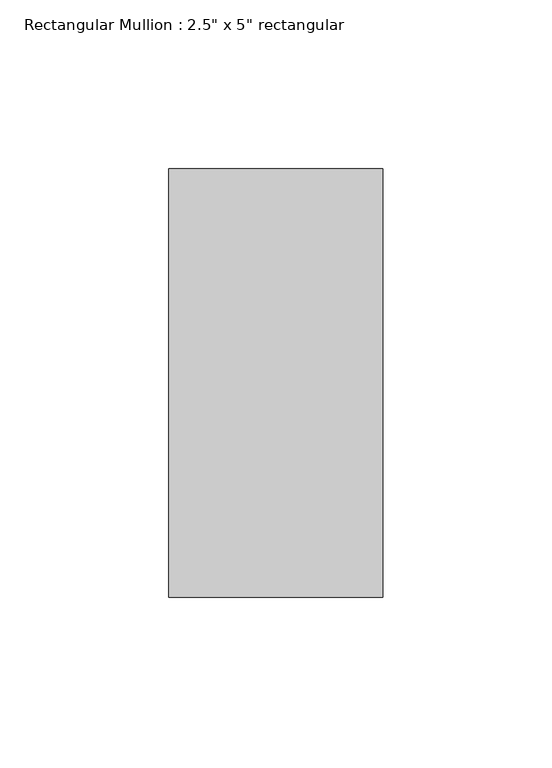
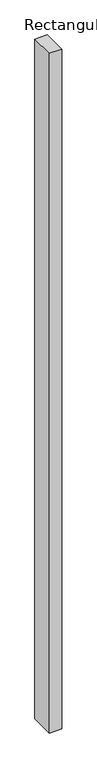
"""IFC4 building model written with IfcOpenShell, lengths in millimetres: member geometry."""

from ifc_helpers import new_model, si_unit, frame, origin, place, context, project, spatial, polyline, outline, extrude, source, transform, mapped, element, save


def member_47c71a51(model_context):
    return source(origin(), model_context, "Body", "SweptSolid", [
        extrude(outline(polyline([(0.0, 63.5), (0.0, -63.5), (-63.5, -63.5), (-63.5, 63.5), (0.0, 63.5)])), frame((0.0, 0.0, -3642.0483533), z_axis=(0.0, 0.0, 1.0), x_axis=(1.0, 0.0, 0.0)), (0.0, 0.0, 1.0), 3642.0483533),
    ])


if __name__ == "__main__":
    model = new_model("IFC4")
    model_context = context("Model", 3, world=origin())
    ifc_project = project(units=[si_unit("LENGTHUNIT", "METRE", prefix="MILLI")], contexts=[model_context])
    site = spatial("IfcSite", under=ifc_project)
    building = spatial("IfcBuilding", under=site)
    placement = place(None, origin())
    member_shape = member_47c71a51(model_context)
    element("IfcMember", 1, ObjectType="Rectangular Mullion : 2.5\" x 5\" rectangular", at=placement, inside=building, context=model_context, shape_type="MappedRepresentation", body=[
        mapped(member_shape, transform((0.0, 0.0, 0.0), x_axis=(1.0, 0.0, 0.0), y_axis=(0.0, 1.0, 0.0), z_axis=(0.0, 0.0, 1.0))),
    ])
    save(model, "model.ifc")

# Revit data of these elements
# Type "Rectangular Mullion : 2.5\" x 5\" rectangular"
#   built-in parameter 1007304 = 0.416667 (stored number, unit not read)
#   built-in parameter 1007301 = 0.104167 (stored number, unit not read)
#   built-in parameter 1007300 = 0.104167 (stored number, unit not read)
# Element 1 (IfcMember, "Rectangular Mullion : 2.5\" x 5\" rectangular")
#   Materials on its faces: "Aluminum"
# Materials
#   "Aluminum": class "Metal", colour RGB 247 247 247, transparency 0, Description = "Aluminum 6061", Cost = 0
